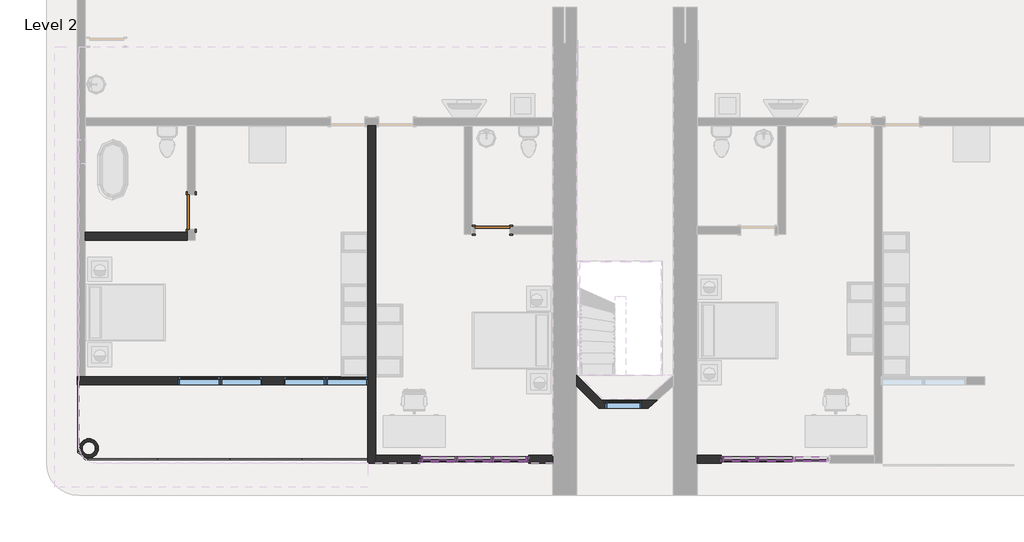
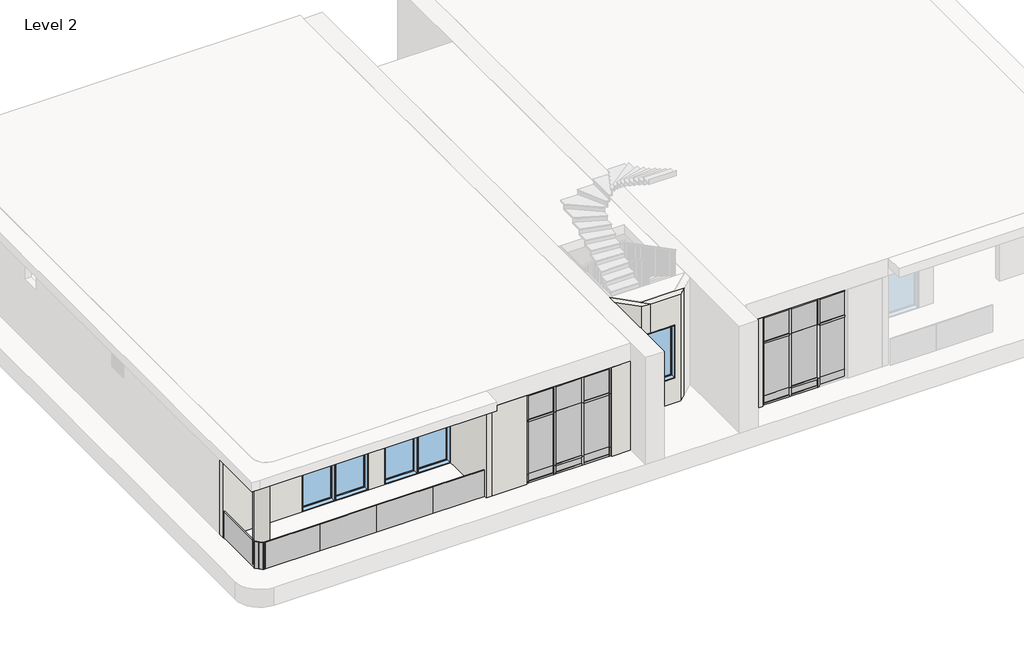
# One storey, part 1 of 5: 37 members, 27 plates, 10 walls, 5 windows, 2 doors.
"""IFC4 building model written with IfcOpenShell, lengths in millimetres."""

from ifc_helpers import new_model, si_unit, point, frame, frame_2d, origin, place, context, project, spatial, polyline, circle_curve, trimmed, segment, composite_curve, outline, extrude, faceted_brep, transform, mapped, element, save
from components import door_2703ae13, member_c17f1be2, member_ad567e07, member_d2e7e466, member_7db1855a, member_75d1e245, member_d60e8053, member_3c3dc66a, member_2fae0574, member_410c6227, member_73c23c35, system_panel_glazed_38d54ecf, system_panel_glazed_fbb6c980, system_panel_glazed_4137532c, system_panel_glazed_6230de04, system_panel_glazed_a79f7f85, system_panel_glazed_9a5ea490, system_panel_glazed_95be5de7, system_panel_glazed_ffe51582, system_panel_glazed_8f95e3f6, system_panel_glazed_836907cd, system_panel_glazed_688a65a2, system_panel_glazed_c1a1c740, system_panel_glazed_22bcd51f, window_9a779fa2, window_1a213a25

model = new_model("IFC4")

# Units and contexts
model_context = context("Model", 3, world=origin())
ifc_project = project(units=[si_unit("LENGTHUNIT", "METRE", prefix="MILLI")], contexts=[model_context])

# Site, building, storey
site = spatial("IfcSite", under=ifc_project)
building = spatial("IfcBuilding", under=site)
storey = spatial("IfcBuildingStorey", under=building, Name="Level 2", Elevation=3657.6)

# Doors
placement = place(None, origin())
door_shape = door_2703ae13(model_context)
element("IfcDoor", 1, ObjectType="Door-Single-Panel.0001 : 34\" x 80\"", at=placement, inside=storey, context=model_context, shape_type="MappedRepresentation", body=[
    mapped(door_shape, transform((-15765.9987704, -441.9241442, 3657.6), x_axis=(0.0, -1.0, 0.0), y_axis=(1.0, 0.0, 0.0), z_axis=(0.0, 0.0, 1.0))),
])
element("IfcDoor", 2, ObjectType="Door-Single-Panel.0001 : 34\" x 80\"", at=placement, inside=storey, context=model_context, shape_type="MappedRepresentation", body=[
    mapped(door_shape, transform((-8145.9987704, -899.1241442, 3657.6), x_axis=(-1.0, 0.0, 0.0), y_axis=(0.0, -1.0, 0.0), z_axis=(0.0, 0.0, 1.0))),
])

# Members
member_shape = member_c17f1be2(model_context)
element("IfcMember", 3, ObjectType="Rectangular Mullion : 2.5\" x 5\" rectangular", at=placement, inside=storey, context=model_context, shape_type="MappedRepresentation", body=[
    mapped(member_shape, transform((-9911.2987704, -6690.3241442, 6705.6), x_axis=(0.0, 0.0, 1.0), y_axis=(0.0, 1.0, 0.0), z_axis=(-1.0, 0.0, 0.0))),
])
element("IfcMember", 4, ObjectType="Rectangular Mullion : 2.5\" x 5\" rectangular", at=placement, inside=storey, context=model_context, shape_type="MappedRepresentation", body=[
    mapped(member_shape, transform((-8114.2487704, -6690.3241442, 6705.6), x_axis=(0.0, 0.0, 1.0), y_axis=(0.0, 1.0, 0.0), z_axis=(-1.0, 0.0, 0.0))),
])
element("IfcMember", 5, ObjectType="Rectangular Mullion : 2.5\" x 5\" rectangular", at=placement, inside=storey, context=model_context, shape_type="MappedRepresentation", body=[
    mapped(member_shape, transform((-2291.2987704, -6690.3241442, 6705.6), x_axis=(0.0, 0.0, 1.0), y_axis=(0.0, 1.0, 0.0), z_axis=(-1.0, 0.0, 0.0))),
])
element("IfcMember", 6, ObjectType="Rectangular Mullion : 2.5\" x 5\" rectangular", at=placement, inside=storey, context=model_context, shape_type="MappedRepresentation", body=[
    mapped(member_shape, transform((-494.2487704, -6690.3241442, 6705.6), x_axis=(0.0, 0.0, 1.0), y_axis=(0.0, 1.0, 0.0), z_axis=(-1.0, 0.0, 0.0))),
])
element("IfcMember", 7, ObjectType="Rectangular Mullion : 2.5\" x 5\" rectangular", at=placement, inside=storey, context=model_context, shape_type="MappedRepresentation", body=[
    mapped(member_shape, transform((-7295.0987704, -6690.3241442, 3657.6), x_axis=(0.0, 0.0, -1.0), y_axis=(0.0, 1.0, 0.0), z_axis=(1.0, 0.0, 0.0))),
])
element("IfcMember", 8, ObjectType="Rectangular Mullion : 2.5\" x 5\" rectangular", at=placement, inside=storey, context=model_context, shape_type="MappedRepresentation", body=[
    mapped(member_shape, transform((-9092.1487704, -6690.3241442, 3657.6), x_axis=(0.0, 0.0, -1.0), y_axis=(0.0, 1.0, 0.0), z_axis=(1.0, 0.0, 0.0))),
])
element("IfcMember", 9, ObjectType="Rectangular Mullion : 2.5\" x 5\" rectangular", at=placement, inside=storey, context=model_context, shape_type="MappedRepresentation", body=[
    mapped(member_shape, transform((-1472.1487704, -6690.3241442, 3657.6), x_axis=(0.0, 0.0, -1.0), y_axis=(0.0, 1.0, 0.0), z_axis=(1.0, 0.0, 0.0))),
])
member_2_shape = member_ad567e07(model_context)
element("IfcMember", 10, ObjectType="Rectangular Mullion : 2.5\" x 5\" rectangular", at=placement, inside=storey, context=model_context, shape_type="MappedRepresentation", body=[
    mapped(member_2_shape, transform((-8114.2487704, -6690.3241442, 5791.2), x_axis=(0.0, 0.0, 1.0), y_axis=(0.0, 1.0, 0.0), z_axis=(-1.0, 0.0, 0.0))),
])
element("IfcMember", 11, ObjectType="Rectangular Mullion : 2.5\" x 5\" rectangular", at=placement, inside=storey, context=model_context, shape_type="MappedRepresentation", body=[
    mapped(member_2_shape, transform((-9911.2987704, -6690.3241442, 5791.2), x_axis=(0.0, 0.0, 1.0), y_axis=(0.0, 1.0, 0.0), z_axis=(-1.0, 0.0, 0.0))),
])
element("IfcMember", 12, ObjectType="Rectangular Mullion : 2.5\" x 5\" rectangular", at=placement, inside=storey, context=model_context, shape_type="MappedRepresentation", body=[
    mapped(member_2_shape, transform((-494.2487704, -6690.3241442, 5791.2), x_axis=(0.0, 0.0, 1.0), y_axis=(0.0, 1.0, 0.0), z_axis=(-1.0, 0.0, 0.0))),
])
element("IfcMember", 13, ObjectType="Rectangular Mullion : 2.5\" x 5\" rectangular", at=placement, inside=storey, context=model_context, shape_type="MappedRepresentation", body=[
    mapped(member_2_shape, transform((-2291.2987704, -6690.3241442, 5791.2), x_axis=(0.0, 0.0, 1.0), y_axis=(0.0, 1.0, 0.0), z_axis=(-1.0, 0.0, 0.0))),
])
member_3_shape = member_d2e7e466(model_context)
element("IfcMember", 14, ObjectType="Rectangular Mullion : 2.5\" x 5\" rectangular", at=placement, inside=storey, context=model_context, shape_type="MappedRepresentation", body=[
    mapped(member_3_shape, transform((-8177.7487704, -6690.3241442, 3657.6), x_axis=(0.0, 0.0, -1.0), y_axis=(0.0, 1.0, 0.0), z_axis=(1.0, 0.0, 0.0))),
])
element("IfcMember", 15, ObjectType="Rectangular Mullion : 2.5\" x 5\" rectangular", at=placement, inside=storey, context=model_context, shape_type="MappedRepresentation", body=[
    mapped(member_3_shape, transform((-557.7487704, -6690.3241442, 3657.6), x_axis=(0.0, 0.0, -1.0), y_axis=(0.0, 1.0, 0.0), z_axis=(1.0, 0.0, 0.0))),
])
member_4_shape = member_7db1855a(model_context)
element("IfcMember", 16, ObjectType="Rectangular Mullion : 2.5\" x 5\" rectangular", at=placement, inside=storey, context=model_context, shape_type="MappedRepresentation", body=[
    mapped(member_4_shape, transform((-9028.6487704, -6690.3241442, 3962.4), x_axis=(0.0, 0.0, 1.0), y_axis=(0.0, 1.0, 0.0), z_axis=(-1.0, 0.0, 0.0))),
])
element("IfcMember", 17, ObjectType="Rectangular Mullion : 2.5\" x 5\" rectangular", at=placement, inside=storey, context=model_context, shape_type="MappedRepresentation", body=[
    mapped(member_4_shape, transform((-1408.6487704, -6690.3241442, 3962.4), x_axis=(0.0, 0.0, 1.0), y_axis=(0.0, 1.0, 0.0), z_axis=(-1.0, 0.0, 0.0))),
])
element("IfcMember", 18, ObjectType="Rectangular Mullion : 2.5\" x 5\" rectangular", at=placement, inside=storey, context=model_context, shape_type="MappedRepresentation", body=[
    mapped(member_3_shape, transform((-9028.6487704, -6690.3241442, 6705.6), x_axis=(0.0, 0.0, 1.0), y_axis=(0.0, 1.0, 0.0), z_axis=(-1.0, 0.0, 0.0))),
])
element("IfcMember", 19, ObjectType="Rectangular Mullion : 2.5\" x 5\" rectangular", at=placement, inside=storey, context=model_context, shape_type="MappedRepresentation", body=[
    mapped(member_3_shape, transform((-1408.6487704, -6690.3241442, 6705.6), x_axis=(0.0, 0.0, 1.0), y_axis=(0.0, 1.0, 0.0), z_axis=(-1.0, 0.0, 0.0))),
])
member_5_shape = member_75d1e245(model_context)
element("IfcMember", 20, ObjectType="Rectangular Mullion : 2.5\" x 5\" rectangular", at=placement, inside=storey, context=model_context, shape_type="MappedRepresentation", body=[
    mapped(member_5_shape, transform((-8145.9987704, -6690.3241442, 3657.6), x_axis=(-1.0, 0.0, 0.0), y_axis=(0.0, 1.0, 0.0), z_axis=(0.0, 0.0, -1.0))),
])
element("IfcMember", 21, ObjectType="Rectangular Mullion : 2.5\" x 5\" rectangular", at=placement, inside=storey, context=model_context, shape_type="MappedRepresentation", body=[
    mapped(member_5_shape, transform((-9060.3987704, -6690.3241442, 3657.6), x_axis=(-1.0, 0.0, 0.0), y_axis=(0.0, 1.0, 0.0), z_axis=(0.0, 0.0, -1.0))),
])
element("IfcMember", 22, ObjectType="Rectangular Mullion : 2.5\" x 5\" rectangular", at=placement, inside=storey, context=model_context, shape_type="MappedRepresentation", body=[
    mapped(member_5_shape, transform((-525.9987704, -6690.3241442, 3657.6), x_axis=(-1.0, 0.0, 0.0), y_axis=(0.0, 1.0, 0.0), z_axis=(0.0, 0.0, -1.0))),
])
element("IfcMember", 23, ObjectType="Rectangular Mullion : 2.5\" x 5\" rectangular", at=placement, inside=storey, context=model_context, shape_type="MappedRepresentation", body=[
    mapped(member_5_shape, transform((-1440.3987704, -6690.3241442, 3657.6), x_axis=(-1.0, 0.0, 0.0), y_axis=(0.0, 1.0, 0.0), z_axis=(0.0, 0.0, -1.0))),
])
member_6_shape = member_d60e8053(model_context)
element("IfcMember", 24, ObjectType="Rectangular Mullion : 2.5\" x 5\" rectangular", at=placement, inside=storey, context=model_context, shape_type="MappedRepresentation", body=[
    mapped(member_6_shape, transform((-8145.9987704, -6690.3241442, 3962.4), x_axis=(-1.0, 0.0, 0.0), y_axis=(0.0, 1.0, 0.0), z_axis=(0.0, 0.0, -1.0))),
])
element("IfcMember", 25, ObjectType="Rectangular Mullion : 2.5\" x 5\" rectangular", at=placement, inside=storey, context=model_context, shape_type="MappedRepresentation", body=[
    mapped(member_6_shape, transform((-9060.3987704, -6690.3241442, 3962.4), x_axis=(-1.0, 0.0, 0.0), y_axis=(0.0, 1.0, 0.0), z_axis=(0.0, 0.0, -1.0))),
])
element("IfcMember", 26, ObjectType="Rectangular Mullion : 2.5\" x 5\" rectangular", at=placement, inside=storey, context=model_context, shape_type="MappedRepresentation", body=[
    mapped(member_6_shape, transform((-1440.3987704, -6690.3241442, 3962.4), x_axis=(-1.0, 0.0, 0.0), y_axis=(0.0, 1.0, 0.0), z_axis=(0.0, 0.0, -1.0))),
])
member_7_shape = member_3c3dc66a(model_context)
element("IfcMember", 27, ObjectType="Rectangular Mullion : 2.5\" x 5\" rectangular", at=placement, inside=storey, context=model_context, shape_type="MappedRepresentation", body=[
    mapped(member_7_shape, transform((-9974.7987704, -6690.3241442, 3657.6), x_axis=(-1.0, 0.0, 0.0), y_axis=(0.0, 1.0, 0.0), z_axis=(0.0, 0.0, -1.0))),
])
element("IfcMember", 28, ObjectType="Rectangular Mullion : 2.5\" x 5\" rectangular", at=placement, inside=storey, context=model_context, shape_type="MappedRepresentation", body=[
    mapped(member_7_shape, transform((-2354.7987704, -6690.3241442, 3657.6), x_axis=(-1.0, 0.0, 0.0), y_axis=(0.0, 1.0, 0.0), z_axis=(0.0, 0.0, -1.0))),
])
member_8_shape = member_2fae0574(model_context)
element("IfcMember", 29, ObjectType="Rectangular Mullion : 2.5\" x 5\" rectangular", at=placement, inside=storey, context=model_context, shape_type="MappedRepresentation", body=[
    mapped(member_8_shape, transform((-9974.7987704, -6690.3241442, 3962.4), x_axis=(-1.0, 0.0, 0.0), y_axis=(0.0, 1.0, 0.0), z_axis=(0.0, 0.0, -1.0))),
])
element("IfcMember", 30, ObjectType="Rectangular Mullion : 2.5\" x 5\" rectangular", at=placement, inside=storey, context=model_context, shape_type="MappedRepresentation", body=[
    mapped(member_8_shape, transform((-2354.7987704, -6690.3241442, 3962.4), x_axis=(-1.0, 0.0, 0.0), y_axis=(0.0, 1.0, 0.0), z_axis=(0.0, 0.0, -1.0))),
])
element("IfcMember", 31, ObjectType="Rectangular Mullion : 2.5\" x 5\" rectangular", at=placement, inside=storey, context=model_context, shape_type="MappedRepresentation", body=[
    mapped(member_8_shape, transform((-7231.5987704, -6690.3241442, 5791.2), x_axis=(1.0, 0.0, 0.0), y_axis=(0.0, 1.0, 0.0), z_axis=(0.0, 0.0, 1.0))),
])
element("IfcMember", 32, ObjectType="Rectangular Mullion : 2.5\" x 5\" rectangular", at=placement, inside=storey, context=model_context, shape_type="MappedRepresentation", body=[
    mapped(member_7_shape, transform((-7231.5987704, -6690.3241442, 3962.4), x_axis=(1.0, 0.0, 0.0), y_axis=(0.0, 1.0, 0.0), z_axis=(0.0, 0.0, 1.0))),
])
member_9_shape = member_410c6227(model_context)
element("IfcMember", 33, ObjectType="Rectangular Mullion : 2.5\" x 5\" rectangular", at=placement, inside=storey, context=model_context, shape_type="MappedRepresentation", body=[
    mapped(member_9_shape, transform((-8145.9987704, -6690.3241442, 5791.2), x_axis=(-1.0, 0.0, 0.0), y_axis=(0.0, 1.0, 0.0), z_axis=(0.0, 0.0, -1.0))),
])
element("IfcMember", 34, ObjectType="Rectangular Mullion : 2.5\" x 5\" rectangular", at=placement, inside=storey, context=model_context, shape_type="MappedRepresentation", body=[
    mapped(member_9_shape, transform((-9060.3987704, -6690.3241442, 5791.2), x_axis=(-1.0, 0.0, 0.0), y_axis=(0.0, 1.0, 0.0), z_axis=(0.0, 0.0, -1.0))),
])
element("IfcMember", 35, ObjectType="Rectangular Mullion : 2.5\" x 5\" rectangular", at=placement, inside=storey, context=model_context, shape_type="MappedRepresentation", body=[
    mapped(member_9_shape, transform((-525.9987704, -6690.3241442, 5791.2), x_axis=(-1.0, 0.0, 0.0), y_axis=(0.0, 1.0, 0.0), z_axis=(0.0, 0.0, -1.0))),
])
element("IfcMember", 36, ObjectType="Rectangular Mullion : 2.5\" x 5\" rectangular", at=placement, inside=storey, context=model_context, shape_type="MappedRepresentation", body=[
    mapped(member_9_shape, transform((-1440.3987704, -6690.3241442, 5791.2), x_axis=(-1.0, 0.0, 0.0), y_axis=(0.0, 1.0, 0.0), z_axis=(0.0, 0.0, -1.0))),
])
member_10_shape = member_73c23c35(model_context)
element("IfcMember", 37, ObjectType="Rectangular Mullion : 2.5\" x 5\" rectangular", at=placement, inside=storey, context=model_context, shape_type="MappedRepresentation", body=[
    mapped(member_10_shape, transform((-7231.5987704, -6690.3241442, 6705.6), x_axis=(1.0, 0.0, 0.0), y_axis=(0.0, 1.0, 0.0), z_axis=(0.0, 0.0, 1.0))),
])
element("IfcMember", 38, ObjectType="Rectangular Mullion : 2.5\" x 5\" rectangular", at=placement, inside=storey, context=model_context, shape_type="MappedRepresentation", body=[
    mapped(member_10_shape, transform((-9974.7987704, -6690.3241442, 5791.2), x_axis=(-1.0, 0.0, 0.0), y_axis=(0.0, 1.0, 0.0), z_axis=(0.0, 0.0, -1.0))),
])
element("IfcMember", 39, ObjectType="Rectangular Mullion : 2.5\" x 5\" rectangular", at=placement, inside=storey, context=model_context, shape_type="MappedRepresentation", body=[
    mapped(member_10_shape, transform((-2354.7987704, -6690.3241442, 5791.2), x_axis=(-1.0, 0.0, 0.0), y_axis=(0.0, 1.0, 0.0), z_axis=(0.0, 0.0, -1.0))),
])

# Plates
system_panel_glazed_shape = system_panel_glazed_38d54ecf(model_context)
element("IfcPlate", 40, ObjectType="System Panel : Glazed", at=placement, inside=storey, context=model_context, shape_type="MappedRepresentation", body=[
    mapped(system_panel_glazed_shape, transform((-8603.1987704, -6690.3241442, 3994.15), x_axis=(-1.0, 0.0, 0.0), y_axis=(0.0, -1.0, 0.0), z_axis=(0.0, 0.0, 1.0))),
])
element("IfcPlate", 41, ObjectType="System Panel : Glazed", at=placement, inside=storey, context=model_context, shape_type="MappedRepresentation", body=[
    mapped(system_panel_glazed_shape, transform((-983.1987704, -6690.3241442, 3994.15), x_axis=(-1.0, 0.0, 0.0), y_axis=(0.0, -1.0, 0.0), z_axis=(0.0, 0.0, 1.0))),
])
system_panel_glazed_2_shape = system_panel_glazed_fbb6c980(model_context)
element("IfcPlate", 42, ObjectType="System Panel : Glazed", at=placement, inside=storey, context=model_context, shape_type="MappedRepresentation", body=[
    mapped(system_panel_glazed_2_shape, transform((-8603.1987704, -6690.3241442, 3721.1), x_axis=(-1.0, 0.0, 0.0), y_axis=(0.0, -1.0, 0.0), z_axis=(0.0, 0.0, 1.0))),
])
element("IfcPlate", 43, ObjectType="System Panel : Glazed", at=placement, inside=storey, context=model_context, shape_type="MappedRepresentation", body=[
    mapped(system_panel_glazed_2_shape, transform((-983.1987704, -6690.3241442, 3721.1), x_axis=(-1.0, 0.0, 0.0), y_axis=(0.0, -1.0, 0.0), z_axis=(0.0, 0.0, 1.0))),
])
system_panel_glazed_3_shape = system_panel_glazed_4137532c(model_context)
element("IfcPlate", 44, ObjectType="System Panel : Glazed", at=placement, inside=storey, context=model_context, shape_type="MappedRepresentation", body=[
    mapped(system_panel_glazed_3_shape, transform((-7704.6737704, -6690.3241442, 3721.1), x_axis=(-1.0, 0.0, 0.0), y_axis=(0.0, -1.0, 0.0), z_axis=(0.0, 0.0, 1.0))),
])
element("IfcPlate", 45, ObjectType="System Panel : Glazed", at=placement, inside=storey, context=model_context, shape_type="MappedRepresentation", body=[
    mapped(system_panel_glazed_3_shape, transform((-9501.7237704, -6690.3241442, 3721.1), x_axis=(-1.0, 0.0, 0.0), y_axis=(0.0, -1.0, 0.0), z_axis=(0.0, 0.0, 1.0))),
])
element("IfcPlate", 46, ObjectType="System Panel : Glazed", at=placement, inside=storey, context=model_context, shape_type="MappedRepresentation", body=[
    mapped(system_panel_glazed_3_shape, transform((-84.6737704, -6690.3241442, 3721.1), x_axis=(-1.0, 0.0, 0.0), y_axis=(0.0, -1.0, 0.0), z_axis=(0.0, 0.0, 1.0))),
])
element("IfcPlate", 47, ObjectType="System Panel : Glazed", at=placement, inside=storey, context=model_context, shape_type="MappedRepresentation", body=[
    mapped(system_panel_glazed_3_shape, transform((-1881.7237704, -6690.3241442, 3721.1), x_axis=(-1.0, 0.0, 0.0), y_axis=(0.0, -1.0, 0.0), z_axis=(0.0, 0.0, 1.0))),
])
system_panel_glazed_4_shape = system_panel_glazed_6230de04(model_context)
element("IfcPlate", 48, ObjectType="System Panel : Glazed", at=placement, inside=storey, context=model_context, shape_type="MappedRepresentation", body=[
    mapped(system_panel_glazed_4_shape, transform((-7704.6737704, -6690.3241442, 3962.4), x_axis=(-1.0, 0.0, 0.0), y_axis=(0.0, -1.0, 0.0), z_axis=(0.0, 0.0, 1.0))),
])
element("IfcPlate", 49, ObjectType="System Panel : Glazed", at=placement, inside=storey, context=model_context, shape_type="MappedRepresentation", body=[
    mapped(system_panel_glazed_4_shape, transform((-9501.7237704, -6690.3241442, 3962.4), x_axis=(-1.0, 0.0, 0.0), y_axis=(0.0, -1.0, 0.0), z_axis=(0.0, 0.0, 1.0))),
])
element("IfcPlate", 50, ObjectType="System Panel : Glazed", at=placement, inside=storey, context=model_context, shape_type="MappedRepresentation", body=[
    mapped(system_panel_glazed_4_shape, transform((-84.6737704, -6690.3241442, 3962.4), x_axis=(-1.0, 0.0, 0.0), y_axis=(0.0, -1.0, 0.0), z_axis=(0.0, 0.0, 1.0))),
])
element("IfcPlate", 51, ObjectType="System Panel : Glazed", at=placement, inside=storey, context=model_context, shape_type="MappedRepresentation", body=[
    mapped(system_panel_glazed_4_shape, transform((-1881.7237704, -6690.3241442, 3962.4), x_axis=(-1.0, 0.0, 0.0), y_axis=(0.0, -1.0, 0.0), z_axis=(0.0, 0.0, 1.0))),
])
system_panel_glazed_5_shape = system_panel_glazed_a79f7f85(model_context)
element("IfcPlate", 52, ObjectType="System Panel : Glazed", at=placement, inside=storey, context=model_context, shape_type="MappedRepresentation", body=[
    mapped(system_panel_glazed_5_shape, transform((-7704.6737704, -6690.3241442, 5822.95), x_axis=(-1.0, 0.0, 0.0), y_axis=(0.0, -1.0, 0.0), z_axis=(0.0, 0.0, 1.0))),
])
element("IfcPlate", 53, ObjectType="System Panel : Glazed", at=placement, inside=storey, context=model_context, shape_type="MappedRepresentation", body=[
    mapped(system_panel_glazed_5_shape, transform((-9501.7237704, -6690.3241442, 5822.95), x_axis=(-1.0, 0.0, 0.0), y_axis=(0.0, -1.0, 0.0), z_axis=(0.0, 0.0, 1.0))),
])
element("IfcPlate", 54, ObjectType="System Panel : Glazed", at=placement, inside=storey, context=model_context, shape_type="MappedRepresentation", body=[
    mapped(system_panel_glazed_5_shape, transform((-84.6737704, -6690.3241442, 5822.95), x_axis=(-1.0, 0.0, 0.0), y_axis=(0.0, -1.0, 0.0), z_axis=(0.0, 0.0, 1.0))),
])
element("IfcPlate", 55, ObjectType="System Panel : Glazed", at=placement, inside=storey, context=model_context, shape_type="MappedRepresentation", body=[
    mapped(system_panel_glazed_5_shape, transform((-1881.7237704, -6690.3241442, 5822.95), x_axis=(-1.0, 0.0, 0.0), y_axis=(0.0, -1.0, 0.0), z_axis=(0.0, 0.0, 1.0))),
])
system_panel_glazed_6_shape = system_panel_glazed_9a5ea490(model_context)
element("IfcPlate", 56, ObjectType="System Panel : Glazed", at=placement, inside=storey, context=model_context, shape_type="MappedRepresentation", body=[
    mapped(system_panel_glazed_6_shape, transform((-8603.1987704, -6690.3241442, 5791.2), x_axis=(-1.0, 0.0, 0.0), y_axis=(0.0, -1.0, 0.0), z_axis=(0.0, 0.0, 1.0))),
])
element("IfcPlate", 57, ObjectType="System Panel : Glazed", at=placement, inside=storey, context=model_context, shape_type="MappedRepresentation", body=[
    mapped(system_panel_glazed_6_shape, transform((-983.1987704, -6690.3241442, 5791.2), x_axis=(-1.0, 0.0, 0.0), y_axis=(0.0, -1.0, 0.0), z_axis=(0.0, 0.0, 1.0))),
])
system_panel_glazed_7_shape = system_panel_glazed_95be5de7(model_context)
element("IfcPlate", 58, ObjectType="System Panel : Glazed", at=placement, inside=storey, context=model_context, shape_type="MappedRepresentation", body=[
    mapped(system_panel_glazed_7_shape, transform((-15707.2305745, -6723.6923401, 3657.6), x_axis=(1.0, 0.0, 0.0), y_axis=(0.0, 1.0, 0.0), z_axis=(0.0, 0.0, 1.0))),
])
element("IfcPlate", 59, ObjectType="System Panel : Glazed", at=placement, inside=storey, context=model_context, shape_type="MappedRepresentation", body=[
    mapped(system_panel_glazed_7_shape, transform((-13878.4305745, -6723.6923401, 3657.6), x_axis=(1.0, 0.0, 0.0), y_axis=(0.0, 1.0, 0.0), z_axis=(0.0, 0.0, 1.0))),
])
system_panel_glazed_8_shape = system_panel_glazed_ffe51582(model_context)
element("IfcPlate", 60, ObjectType="System Panel : Glazed", at=placement, inside=storey, context=model_context, shape_type="MappedRepresentation", body=[
    mapped(system_panel_glazed_8_shape, transform((-18451.9713429, -6722.1515718, 3657.6), x_axis=(0.7071067811865462, -0.7071067811865488, 0.0), y_axis=(0.7071067811865488, 0.7071067811865462, 0.0), z_axis=(0.0, 0.0, 1.0))),
])
system_panel_glazed_9_shape = system_panel_glazed_8f95e3f6(model_context)
element("IfcPlate", 61, ObjectType="System Panel : Glazed", at=placement, inside=storey, context=model_context, shape_type="MappedRepresentation", body=[
    mapped(system_panel_glazed_9_shape, transform((-18648.8987704, -5667.9741442, 3657.6), x_axis=(0.0, -1.0, 0.0), y_axis=(1.0, 0.0, 0.0), z_axis=(0.0, 0.0, 1.0))),
])
system_panel_glazed_10_shape = system_panel_glazed_836907cd(model_context)
element("IfcPlate", 62, ObjectType="System Panel : Glazed", at=placement, inside=storey, context=model_context, shape_type="MappedRepresentation", body=[
    mapped(system_panel_glazed_10_shape, transform((-18418.6805745, -6723.6923401, 3657.6), x_axis=(1.0, 0.0, 0.0), y_axis=(0.0, 1.0, 0.0), z_axis=(0.0, 0.0, 1.0))),
])
system_panel_glazed_11_shape = system_panel_glazed_688a65a2(model_context)
element("IfcPlate", 63, ObjectType="System Panel : Glazed", at=placement, inside=storey, context=model_context, shape_type="MappedRepresentation", body=[
    mapped(system_panel_glazed_11_shape, transform((-12129.8146725, -6723.6923401, 3657.6), x_axis=(1.0, 0.0, 0.0), y_axis=(0.0, 1.0, 0.0), z_axis=(0.0, 0.0, 1.0))),
])
system_panel_glazed_12_shape = system_panel_glazed_c1a1c740(model_context)
element("IfcPlate", 64, ObjectType="System Panel : Glazed", at=placement, inside=storey, context=model_context, shape_type="MappedRepresentation", body=[
    mapped(system_panel_glazed_12_shape, transform((-17504.2805745, -6723.6923401, 3657.6), x_axis=(1.0, 0.0, 0.0), y_axis=(0.0, 1.0, 0.0), z_axis=(0.0, 0.0, 1.0))),
])
system_panel_glazed_13_shape = system_panel_glazed_22bcd51f(model_context)
element("IfcPlate", 65, ObjectType="System Panel : Glazed", at=placement, inside=storey, context=model_context, shape_type="MappedRepresentation", body=[
    mapped(system_panel_glazed_13_shape, transform((-18600.0521056, -6574.070809, 3657.6), x_axis=(0.7071067811865462, -0.7071067811865488, 0.0), y_axis=(0.7071067811865488, 0.7071067811865462, 0.0), z_axis=(0.0, 0.0, 1.0))),
])
element("IfcPlate", 66, ObjectType="System Panel : Glazed", at=placement, inside=storey, context=model_context, shape_type="MappedRepresentation", body=[
    mapped(system_panel_glazed_13_shape, transform((-18502.3587761, -6671.7641386, 3657.6), x_axis=(0.7071067811865462, -0.7071067811865488, 0.0), y_axis=(0.7071067811865488, 0.7071067811865462, 0.0), z_axis=(0.0, 0.0, 1.0))),
])

# Walls
element("IfcWall", 67, ObjectType="Generic - 3\" green 2", at=placement, inside=storey, context=model_context, shape_type="SweptSolid", body=[
    extrude(outline(composite_curve([segment(polyline([(-18518.7237704, -6418.8616442), (-18594.9237704, -6418.8616442)]), True, "CONTINUOUS"), segment(trimmed(circle_curve(frame_2d((-18353.6237704, -6418.8616442)), 241.3), [point((-18594.9237704, -6418.8616442))], [point((-18112.3237704, -6418.8616442))], False, "CARTESIAN"), True, "CONTINUOUS"), segment(polyline([(-18112.3237704, -6418.8616442), (-18188.5237704, -6418.8616442)]), True, "CONTINUOUS"), segment(trimmed(circle_curve(frame_2d((-18353.6237704, -6418.8616442)), 165.1), [point((-18188.5237704, -6418.8616442))], [point((-18518.7237704, -6418.8616442))], True, "CARTESIAN"), True, "CONTINUOUS")], self_intersect=False)), frame((0.0, 0.0, 3657.6), z_axis=(0.0, 0.0, 1.0), x_axis=(1.0, 0.0, 0.0)), (0.0, 0.0, 1.0), 3048.0),
])
element("IfcWall", 68, ObjectType="Generic - 3\" green 2", at=placement, inside=storey, context=model_context, shape_type="SweptSolid", body=[
    extrude(outline(composite_curve([segment(polyline([(-18188.5237704, -6418.8616442), (-18112.3237704, -6418.8616442)]), True, "CONTINUOUS"), segment(trimmed(circle_curve(frame_2d((-18353.6237704, -6418.8616442)), 241.3), [point((-18112.3237704, -6418.8616442))], [point((-18594.9237704, -6418.8616442))], False, "CARTESIAN"), True, "CONTINUOUS"), segment(polyline([(-18594.9237704, -6418.8616442), (-18518.7237704, -6418.8616442)]), True, "CONTINUOUS"), segment(trimmed(circle_curve(frame_2d((-18353.6237704, -6418.8616442)), 165.1), [point((-18518.7237704, -6418.8616442))], [point((-18188.5237704, -6418.8616442))], True, "CARTESIAN"), True, "CONTINUOUS")], self_intersect=False)), frame((0.0, 0.0, 3657.6), z_axis=(0.0, 0.0, 1.0), x_axis=(1.0, 0.0, 0.0)), (0.0, 0.0, 1.0), 3048.0),
])
element("IfcWall", 69, ObjectType="Generic - 8\" cream", at=placement, inside=storey, context=model_context, shape_type="Brep", body=[
    faceted_brep([(-11295.5987704, 1742.4758558, 3657.6), (-11295.5987704, -4607.5241442, 3657.6), (-11295.5987704, -4810.7241442, 3657.6), (-11295.5987704, -6791.9241442, 3657.6), (-11295.5987704, -6791.9241442, 6705.6), (-11295.5987704, -4810.7241442, 6705.6), (-11295.5987704, -4607.5241442, 6705.6), (-11295.5987704, 1742.4758558, 6705.6), (-11092.3987704, 1742.4758558, 3657.6), (-11092.3987704, 1742.4758558, 6705.6), (-11092.3987704, -6588.7241442, 6705.6), (-11092.3987704, -6791.9241442, 6705.6), (-11092.3987704, -6791.9241442, 3657.6), (-11092.3987704, -6588.7241442, 3657.6)], [[[0, 1, 2, 3, 4, 5, 6, 7]], [[8, 9, 10, 11, 12, 13]], [[3, 2, 1, 0, 8, 13, 12]], [[7, 6, 5, 4, 11, 10, 9]], [[0, 7, 9, 8]], [[4, 3, 12, 11]]]),
])
element("IfcWall", 70, ObjectType="Generic - 8\" cream", at=placement, inside=storey, context=model_context, shape_type="SweptSolid", body=[
    extrude(outline(polyline([(-18445.6987704, -949.9241442), (-15867.5987704, -949.9241442), (-15867.5987704, -1153.1241442), (-18445.6987704, -1153.1241442), (-18445.6987704, -949.9241442)])), frame((0.0, 0.0, 3657.6), z_axis=(0.0, 0.0, 1.0), x_axis=(1.0, 0.0, 0.0)), (0.0, 0.0, 1.0), 3048.0),
])
element("IfcWall", 71, ObjectType="Generic - 8\" cream", at=placement, inside=storey, context=model_context, shape_type="Brep", body=[
    faceted_brep([(-18648.8987704, -4607.5241442, 6705.6), (-18445.6987704, -4607.5241442, 6705.6), (-11295.5987704, -4607.5241442, 6705.6), (-11295.5987704, -4607.5241442, 6400.8), (-13429.1987704, -4607.5241442, 6400.8), (-13429.1987704, -4607.5241442, 3657.6), (-13962.5987704, -4607.5241442, 3657.6), (-13962.5987704, -4607.5241442, 6400.8), (-16096.1987704, -4607.5241442, 6400.8), (-16096.1987704, -4607.5241442, 3657.6), (-18445.6987704, -4607.5241442, 3657.6), (-18648.8987704, -4607.5241442, 3657.6), (-11295.5987704, -4810.7241442, 6705.6), (-18648.8987704, -4810.7241442, 6705.6), (-18648.8987704, -4810.7241442, 3657.6), (-16096.1987704, -4810.7241442, 3657.6), (-16096.1987704, -4810.7241442, 6400.8), (-13962.5987704, -4810.7241442, 6400.8), (-13962.5987704, -4810.7241442, 3657.6), (-13429.1987704, -4810.7241442, 3657.6), (-13429.1987704, -4810.7241442, 6400.8), (-11295.5987704, -4810.7241442, 6400.8)], [[[0, 1, 2, 3, 4, 5, 6, 7, 8, 9, 10, 11]], [[12, 13, 14, 15, 16, 17, 18, 19, 20, 21]], [[14, 11, 10, 9, 15]], [[5, 19, 18, 6]], [[2, 1, 0, 13, 12]], [[2, 12, 21, 3]], [[0, 11, 14, 13]], [[3, 21, 20, 4]], [[4, 20, 19, 5]], [[17, 7, 6, 18]], [[7, 17, 16, 8]], [[8, 16, 15, 9]]]),
])
element("IfcWall", 72, ObjectType="Generic - 8\" cream", at=placement, inside=storey, context=model_context, shape_type="SweptSolid", body=[
    extrude(outline(polyline([(-2354.7987704, -6791.9241442), (-2964.3987704, -6791.9241442), (-2964.3987704, -6588.7241442), (-2354.7987704, -6588.7241442), (-2354.7987704, -6791.9241442)])), frame((0.0, 0.0, 3657.6), z_axis=(0.0, 0.0, 1.0), x_axis=(1.0, 0.0, 0.0)), (0.0, 0.0, 1.0), 3048.0),
])
element("IfcWall", 73, ObjectType="Generic - 8\" cream", at=placement, inside=storey, context=model_context, shape_type="SweptSolid", body=[
    extrude(outline(polyline([(-9974.7987704, -6791.9241442), (-11092.3987704, -6791.9241442), (-11092.3987704, -6588.7241442), (-9974.7987704, -6588.7241442), (-9974.7987704, -6791.9241442)])), frame((0.0, 0.0, 3657.6), z_axis=(0.0, 0.0, 1.0), x_axis=(1.0, 0.0, 0.0)), (0.0, 0.0, 1.0), 3048.0),
])
element("IfcWall", 74, ObjectType="Generic - 8\" cream", at=placement, inside=storey, context=model_context, shape_type="SweptSolid", body=[
    extrude(outline(polyline([(-7231.5987704, -6588.7241442), (-6621.9987704, -6588.7241442), (-6621.9987704, -6791.9241442), (-7231.5987704, -6791.9241442), (-7231.5987704, -6588.7241442)])), frame((0.0, 0.0, 3657.6), z_axis=(0.0, 0.0, 1.0), x_axis=(1.0, 0.0, 0.0)), (0.0, 0.0, 1.0), 3048.0),
])
element("IfcWall", 75, ObjectType="Generic - 8\" green", at=placement, inside=storey, context=model_context, shape_type="Brep", body=[
    faceted_brep([(-6012.3987704, -4852.8082422, 3657.6), (-5458.7044276, -5406.502585, 3657.6), (-5458.7044276, -5406.502585, 7315.2), (-6012.3987704, -4852.8082422, 7315.2), (-5171.3362318, -5406.502585, 3657.6), (-5374.5362318, -5203.302585, 3657.6), (-6012.3987704, -4565.4400463, 3657.6), (-6012.3987704, -4565.4400463, 7315.2), (-5374.5362318, -5203.302585, 7315.2), (-5171.3362318, -5406.502585, 7315.2), (-5171.3362318, -5406.502585, 6324.6), (-5289.4901401, -5288.3486766, 6324.6), (-5289.4901401, -5288.3486766, 4495.8), (-5171.3362318, -5406.502585, 4495.8), (-5289.4901401, -5406.502585, 4495.8), (-5289.4901401, -5406.502585, 6324.6)], [[[0, 1, 2, 3]], [[4, 5, 6, 7, 8, 9, 10, 11, 12, 13]], [[1, 0, 6, 5, 4]], [[3, 2, 9, 8, 7]], [[0, 3, 7, 6]], [[2, 1, 4, 13, 14, 15, 10, 9]], [[12, 14, 13]], [[14, 12, 11, 15]], [[15, 11, 10]]]),
])
element("IfcWall", 76, ObjectType="Generic - 8\" green", at=placement, inside=storey, context=model_context, shape_type="Brep", body=[
    faceted_brep([(-5171.3362318, -5406.502585, 3657.6), (-4203.3343712, -5406.502585, 3657.6), (-4203.3343712, -5406.502585, 7315.2), (-5171.3362318, -5406.502585, 7315.2), (-5171.3362318, -5406.502585, 6324.6), (-4375.0901401, -5406.502585, 6324.6), (-4375.0901401, -5406.502585, 4495.8), (-5171.3362318, -5406.502585, 4495.8), (-3975.4820774, -5203.302585, 3657.6), (-4280.7801413, -5203.302585, 3657.6), (-5374.5362318, -5203.302585, 3657.6), (-5374.5362318, -5203.302585, 7315.2), (-4280.7801413, -5203.302585, 7315.2), (-3975.4820774, -5203.302585, 7315.2), (-4375.0901401, -5203.302585, 4495.8), (-4375.0901401, -5203.302585, 6324.6), (-5289.4901401, -5203.302585, 6324.6), (-5289.4901401, -5203.302585, 4495.8), (-5289.4901401, -5288.3486766, 4495.8), (-5289.4901401, -5288.3486766, 6324.6)], [[[0, 1, 2, 3, 4, 5, 6, 7]], [[8, 9, 10, 11, 12, 13], [14, 15, 16, 17]], [[1, 0, 10, 9, 8]], [[3, 2, 13, 12, 11]], [[3, 11, 10, 0, 7, 18, 19, 4]], [[2, 1, 8, 13]], [[5, 15, 14, 6]], [[6, 14, 17, 18, 7]], [[18, 17, 16, 19]], [[15, 5, 4, 19, 16]]]),
])

# Windows
window_shape = window_9a779fa2(model_context)
element("IfcWindow", 77, ObjectType="Fixed : 36\" x 72\"", at=placement, inside=storey, context=model_context, shape_type="MappedRepresentation", body=[
    mapped(window_shape, transform((-4794.1901401, -5304.902585, 4191.0), x_axis=(1.0, 0.0, 0.0), y_axis=(0.0, 1.0, 0.0), z_axis=(0.0, 0.0, 1.0))),
])
window_2_shape = window_1a213a25(model_context)
element("IfcWindow", 78, ObjectType="Fixed : 36\" x 72\" 2", at=placement, inside=storey, context=model_context, shape_type="MappedRepresentation", body=[
    mapped(window_2_shape, transform((-11790.8987704, -4709.1241442, 3352.8), x_axis=(1.0, 0.0, 0.0), y_axis=(0.0, 1.0, 0.0), z_axis=(0.0, 0.0, 1.0))),
])
element("IfcWindow", 79, ObjectType="Fixed : 36\" x 72\" 2", at=placement, inside=storey, context=model_context, shape_type="MappedRepresentation", body=[
    mapped(window_2_shape, transform((-12857.6987704, -4709.1241442, 3352.8), x_axis=(1.0, 0.0, 0.0), y_axis=(0.0, 1.0, 0.0), z_axis=(0.0, 0.0, 1.0))),
])
element("IfcWindow", 80, ObjectType="Fixed : 36\" x 72\" 2", at=placement, inside=storey, context=model_context, shape_type="MappedRepresentation", body=[
    mapped(window_2_shape, transform((-14457.8987704, -4709.1241442, 3352.8), x_axis=(1.0, 0.0, 0.0), y_axis=(0.0, 1.0, 0.0), z_axis=(0.0, 0.0, 1.0))),
])
element("IfcWindow", 81, ObjectType="Fixed : 36\" x 72\" 2", at=placement, inside=storey, context=model_context, shape_type="MappedRepresentation", body=[
    mapped(window_2_shape, transform((-15524.6987704, -4709.1241442, 3352.8), x_axis=(1.0, 0.0, 0.0), y_axis=(0.0, 1.0, 0.0), z_axis=(0.0, 0.0, 1.0))),
])

save(model, "model.ifc")

# Revit data of these elements
# Type "Door-Single-Panel.0001 : 34\" x 80\""
#   Type Mark = "9"
#   Construction Type Id = "DOOR"
#   Assembly Code = "C1020300"
#   Analytic Construction = "Wooden"
#   Thickness = 0' - 2"
#   Thermal Resistance (R) = 0.455703 (m²·K)/W
#   Swing Angle [instance default] = 90.00°
#   Heat Transfer Coefficient (U) = 2.19465 W/(m²·K)
#   Height = 6' - 8"
#   Trim Projection Ext = 0' - 1"
#   Trim Projection Int = 0' - 1"
#   Trim Width = 0' - 3"
#   Width = 2' - 10"
#   Panel Material = Wood - Birch - Solid Stained Light Low Gloss
#   Trim Material = Paint - Sienna
#   Visual Light Transmittance = 0
#   Solar Heat Gain Coefficient = 0
#   Function = (empty or 0)
#   Wall Closure = (empty or 0)
# Type "Rectangular Mullion : 2.5\" x 5\" rectangular"
#   built-in parameter 1007304 = 0.416667 (stored number, unit not read)
#   built-in parameter 1007301 = 0.104167 (stored number, unit not read)
#   built-in parameter 1007300 = 0.104167 (stored number, unit not read)
# Type "System Panel : Glazed"
#   Construction Type Id = "GSP4R"
#   Analytic Construction = "1/8 in Pilkington single glazing"
#   Visual Light Transmittance = 0.9
#   Solar Heat Gain Coefficient = 0.86
#   Heat Transfer Coefficient (U) = 6.7069 W/(m²·K)
# Type "Generic - 3\" green 2"
#   Assembly Code = "B2010"
#   Width = 0' - 3"
#   Layers, outside or top first: 0' - 3" "Damp-proofing" (function 1)
# Type "Generic - 8\" cream"
#   Assembly Code = "B2010"
#   Width = 0' - 8"
#   Layers, outside or top first: 0' - 8" "Parking Stripe" (function 1)
# Type "Generic - 8\" green"
#   Assembly Code = "B2010"
#   Width = 0' - 8"
#   Layers, outside or top first: 0' - 8" "Damp-proofing" (function 1)
# Type "Fixed : 36\" x 72\""
#   Type Mark = "9"
#   Construction Type Id = "GSP4R"
#   Assembly Code = "B2020100"
#   Analytic Construction = "1/8 in Pilkington single glazing"
#   Visual Light Transmittance = 0.9
#   Solar Heat Gain Coefficient = 0.78
#   Heat Transfer Coefficient (U) = 3.6886 W/(m²·K)
#   Height = 6' - 0"
#   Default Sill Height = 1' - 0"
#   Width = 3' - 0"
#   Window Inset = 0' - 0 3/4"
#   Glass Pane Material = Glass
#   Sash Material = Iron, Ductile
#   Wall Closure = (empty or 0)
# Type "Fixed : 36\" x 72\" 2"
#   Type Mark = "29"
#   Construction Type Id = "GSP4R"
#   Assembly Code = "B2020100"
#   Analytic Construction = "1/8 in Pilkington single glazing"
#   Visual Light Transmittance = 0.9
#   Solar Heat Gain Coefficient = 0.78
#   Heat Transfer Coefficient (U) = 3.6886 W/(m²·K)
#   Height = 9' - 0"
#   Default Sill Height = 1' - 0"
#   Width = 3' - 6"
#   Window Inset = 0' - 0 3/4"
#   Glass Pane Material = Glass
#   Sash Material = Iron, Ductile
#   Wall Closure = (empty or 0)
# Elements 1, 2 (IfcDoor, "Door-Single-Panel.0001 : 34\" x 80\"")
#   Swing Angle = 90.00°
#   Phase Created = New Construction
#   Materials on its faces: "Paint - Sienna", "Wood - Birch - Solid Stained Light Low Gloss"
# Elements 3, 4, 5, 6, 7, 8, 9, 10, 11, 12, 13, 14, 15, 16, 17, 18, 19, 20, 21, 22, 23, 24, 25, 26, 27, 28, 29, 30, 31, 32, 33, 34, 35, 36, 37, 38, 39 (IfcMember, "Rectangular Mullion : 2.5\" x 5\" rectangular")
#   Phase Created = New Construction
#   Materials on its faces: "Iron, Ductile"
# Elements 40, 41, 42, 43, 44, 45, 46, 47, 48, 49, 50, 51, 52, 53, 54, 55, 56, 57, 58, 59, 60, 61, 62, 63, 64, 65, 66 (IfcPlate, "System Panel : Glazed")
#   Phase Created = New Construction
#   Materials on its faces: "Glass"
# Elements 67, 68 (IfcWall, "Generic - 3\" green 2")
#   Top Offset = 0' - 0"
#   Base Offset = 0' - 0"
#   Unconnected Height = 10' - 0"
#   wall height = 10' - 0"
#   Phase Created = New Construction
#   Materials on its faces: "Damp-proofing"
# Elements 69, 70, 71, 72, 73, 74 (IfcWall, "Generic - 8\" cream")
#   Top Offset = 0' - 0"
#   Base Offset = 0' - 0"
#   Unconnected Height = 10' - 0"
#   wall height = 10' - 0"
#   Phase Created = New Construction
#   Base Constraint = Level 2
#   Materials on its faces: "Parking Stripe"
# Elements 75, 76 (IfcWall, "Generic - 8\" green")
#   Top Offset = 0' - 0"
#   Base Offset = 0' - 0"
#   Unconnected Height = 12' - 0"
#   wall height = 12' - 0"
#   Phase Created = New Construction
#   Base Constraint = Level 2
#   Materials on its faces: "Damp-proofing"
# Element 77 (IfcWindow, "Fixed : 36\" x 72\"")
#   Mark = "13"
#   Phase Created = New Construction
#   Materials on its faces: "Iron, Ductile", "Glass"
# Element 78 (IfcWindow, "Fixed : 36\" x 72\" 2")
#   Mark = "14"
#   Phase Created = New Construction
#   Materials on its faces: "Iron, Ductile", "Glass"
# Element 79 (IfcWindow, "Fixed : 36\" x 72\" 2")
#   Mark = "15"
#   Phase Created = New Construction
#   Materials on its faces: "Iron, Ductile", "Glass"
# Element 80 (IfcWindow, "Fixed : 36\" x 72\" 2")
#   Mark = "16"
#   Phase Created = New Construction
#   Materials on its faces: "Iron, Ductile", "Glass"
# Element 81 (IfcWindow, "Fixed : 36\" x 72\" 2")
#   Mark = "17"
#   Phase Created = New Construction
#   Materials on its faces: "Iron, Ductile", "Glass"
# Materials
#   "Wood - Birch - Solid Stained Light Low Gloss": class "Wood", colour RGB 210 159 95, transparency 0, Cost = 0
#   "Paint - Sienna": colour RGB 118 70 51, transparency 0, Cost = 0
#   "Damp-proofing": class "Generic", colour RGB 127 127 127, transparency 0, Description = "Damp-proofing", Cost = 0
#   "Parking Stripe": class "Paint", colour RGB 250 250 91, transparency 0, Cost = 0
#   "Glass": class "Glass", colour RGB 0 128 192, transparency 0.75, Description = "Soda Lime Glass", Cost = 0
#   "Iron, Ductile": class "Metal", colour RGB 0 0 0, transparency 0, Description = "Ductile cast iron", Cost = 0
